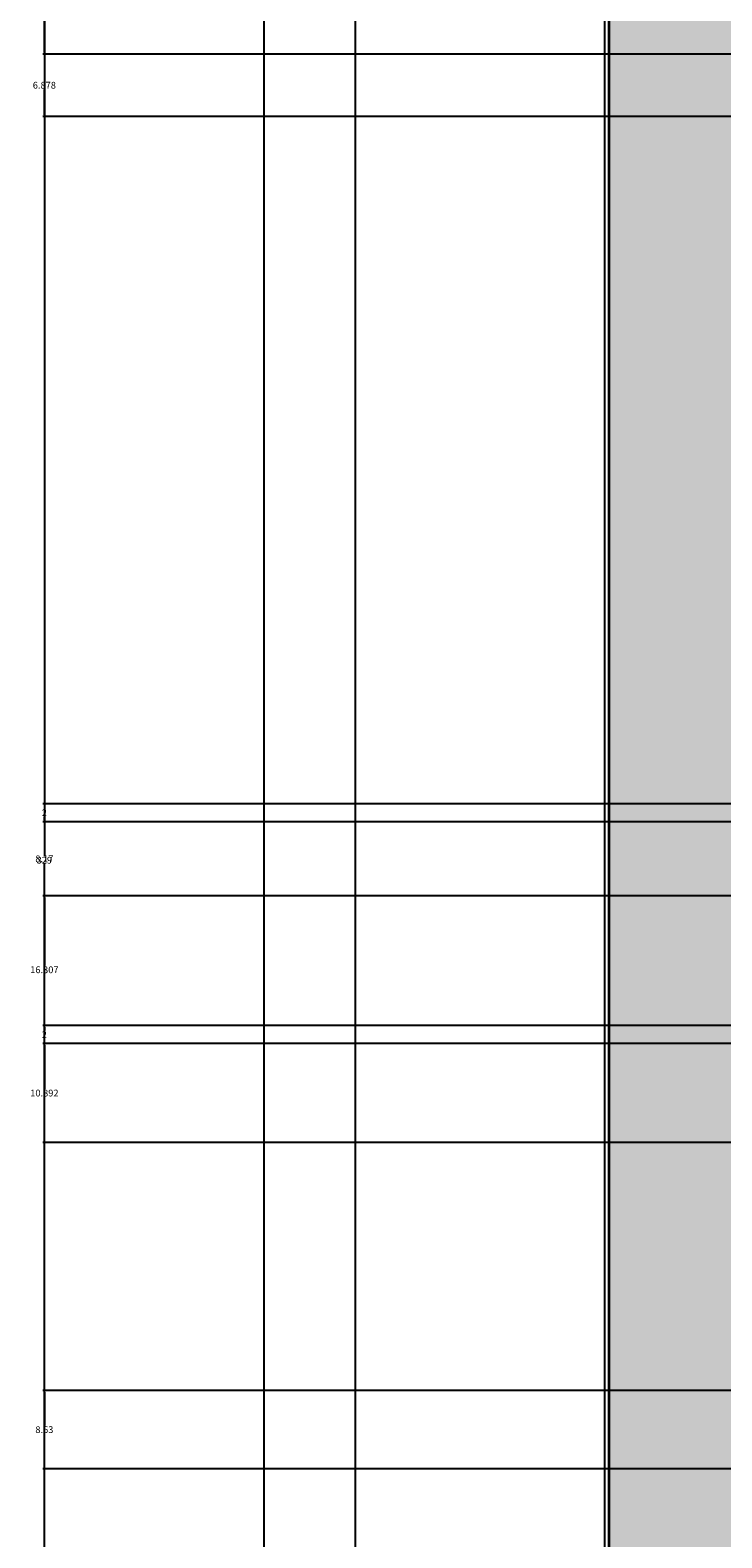
# Model space of a CAD drawing. Units: inches. Extents: x 62 to 566, y 66 to 528.
# Tile 5 of 20: x 62 to 138, y 264 to 430. Entities that reach past the tile are written whole.
import ezdxf

# ---------------------------------------------------------------- set-up
doc = ezdxf.new("R2010")
doc.units = ezdxf.units.IN
doc.header["$MEASUREMENT"] = 0
for name, color, linetype, lineweight in [('A-ANNO-DIMS', 2, 'Continuous', 18), ('A-ELEV', 7, 'Continuous', 35), ('A-WALL-PATT', 8, 'Continuous', 13)]:
    doc.layers.add(name, color=color, linetype=linetype, lineweight=lineweight)
doc.styles.get("Standard").update_dxf_attribs({"font": 'arial.ttf'})
doc.dimstyles.get("Standard").update_dxf_attribs({"dimtxt": 0.75, "dimasz": 0.18, "dimexe": 0.18, "dimexo": 0.0625, "dimgap": 0.09, "dimtad": 0, "dimtih": 1, "dimtoh": 1, "dimdec": 4, "dimzin": 0, "dimdsep": 46, "dimlunit": 4, "dimtxsty": 'Standard', "dimcen": 0.09, "dimadec": 0, "dimazin": 0, "dimtfac": 1, "dimtdec": 4, "dimtofl": 0, "dimtmove": 0, "dimatfit": 3, "dimfxl": 1, "dimtolj": 1, "dimtzin": 0, "dimarcsym": 0})

# ---------------------------------------------------------------- blocks, each defined once
blk = doc.blocks.new('*D8')
at = {"layer": 'A-ANNO-DIMS', "color": 0, "lineweight": -2, "transparency": 16777216}
for p, q in [((284.2, 271.35), (284.2, 65.94)), ((125.94, 126.31), (125.94, 65.94)), ((126.12, 66.12), (203.46, 66.12)), ((284.02, 66.12), (206.68, 66.12))]:
    blk.add_line(p, q, dxfattribs=at)
at = {"layer": 'A-ANNO-DIMS', "color": 0, "transparency": 16777216}
for points in [[(126.12, 66.15), (126.12, 66.09), (125.94, 66.12)], [(284.02, 66.15), (284.02, 66.09), (284.2, 66.12)]]:
    blk.add_solid(points, dxfattribs=at)
at = {"layer": 'Defpoints', "color": 0, "transparency": 16777216}
for p in [(284.2, 271.41), (125.94, 126.37), (284.2, 66.12)]:
    blk.add_point(p, dxfattribs=at)
at = {"layer": 'A-ANNO-DIMS', "color": 0, "transparency": 16777216, "insert": (205.07, 66.12), "char_height": 0.75, "attachment_point": 5}
blk.add_mtext('\\A1;158.26', dxfattribs=at)
blk = doc.blocks.new('*D14')
at = {"layer": 'A-ANNO-DIMS', "color": 0, "lineweight": -2, "transparency": 16777216}
for p, q in [((87.9, 174.13), (87.9, 527.47)), ((88.08, 527.29), (91.61, 527.29)), ((97.79, 527.29), (94.25, 527.29)), ((97.97, 174.13), (97.97, 527.47))]:
    blk.add_line(p, q, dxfattribs=at)
at = {"layer": 'A-ANNO-DIMS', "color": 0, "transparency": 16777216}
for points in [[(88.08, 527.32), (88.08, 527.26), (87.9, 527.29)], [(97.79, 527.32), (97.79, 527.26), (97.97, 527.29)]]:
    blk.add_solid(points, dxfattribs=at)
at = {"layer": 'Defpoints', "color": 0, "transparency": 16777216}
for p in [(97.97, 527.29), (87.9, 174.07), (97.97, 174.07)]:
    blk.add_point(p, dxfattribs=at)
at = {"layer": 'A-ANNO-DIMS', "color": 0, "transparency": 16777216, "insert": (92.93, 527.29), "char_height": 0.75, "attachment_point": 5}
blk.add_mtext('\\A1;10.07', dxfattribs=at)
blk = doc.blocks.new('*D15')
at = {"layer": 'A-ANNO-DIMS', "color": 0, "lineweight": -2, "transparency": 16777216}
for p, q in [((97.97, 174.13), (97.97, 527.47)), ((98.15, 527.29), (110.64, 527.29)), ((125.28, 527.29), (112.79, 527.29)), ((125.46, 174.13), (125.46, 527.47))]:
    blk.add_line(p, q, dxfattribs=at)
at = {"layer": 'A-ANNO-DIMS', "color": 0, "transparency": 16777216}
for points in [[(98.15, 527.32), (98.15, 527.26), (97.97, 527.29)], [(125.28, 527.32), (125.28, 527.26), (125.46, 527.29)]]:
    blk.add_solid(points, dxfattribs=at)
at = {"layer": 'Defpoints', "color": 0, "transparency": 16777216}
for p in [(125.46, 527.29), (97.97, 174.07), (125.46, 174.07)]:
    blk.add_point(p, dxfattribs=at)
at = {"layer": 'A-ANNO-DIMS', "color": 0, "transparency": 16777216, "insert": (111.72, 527.29), "char_height": 0.75, "attachment_point": 5}
blk.add_mtext('\\A1;27.5', dxfattribs=at)
blk = doc.blocks.new('*D18')
at = {"layer": 'A-ANNO-DIMS', "color": 0, "lineweight": -2, "transparency": 16777216}
for p, q in [((120.34, 503.04), (63.47, 503.04)), ((63.65, 502.86), (63.65, 339.03)), ((63.65, 174.25), (63.65, 338.08)), ((87.83, 174.07), (63.47, 174.07))]:
    blk.add_line(p, q, dxfattribs=at)
at = {"layer": 'A-ANNO-DIMS', "color": 0, "transparency": 16777216}
for points in [[(63.62, 502.86), (63.68, 502.86), (63.65, 503.04)], [(63.62, 174.25), (63.68, 174.25), (63.65, 174.07)]]:
    blk.add_solid(points, dxfattribs=at)
at = {"layer": 'Defpoints', "color": 0, "transparency": 16777216}
for p in [(63.65, 503.04), (120.41, 503.04), (87.9, 174.07)]:
    blk.add_point(p, dxfattribs=at)
at = {"layer": 'A-ANNO-DIMS', "color": 0, "transparency": 16777216, "insert": (63.65, 338.55), "char_height": 0.75, "attachment_point": 5}
blk.add_mtext('\\A1;329', dxfattribs=at)
blk = doc.blocks.new('*D35')
at = {"layer": 'A-ANNO-DIMS', "color": 0, "lineweight": -2, "transparency": 16777216}
for p, q in [((125.94, 461.98), (125.94, 65.94)), ((142.39, 445.04), (142.39, 65.94)), ((126.12, 66.12), (132.55, 66.12)), ((142.21, 66.12), (135.77, 66.12))]:
    blk.add_line(p, q, dxfattribs=at)
at = {"layer": 'A-ANNO-DIMS', "color": 0, "transparency": 16777216}
for points in [[(126.12, 66.15), (126.12, 66.09), (125.94, 66.12)], [(142.21, 66.15), (142.21, 66.09), (142.39, 66.12)]]:
    blk.add_solid(points, dxfattribs=at)
at = {"layer": 'Defpoints', "color": 0, "transparency": 16777216}
for p in [(125.94, 462.04), (142.39, 445.11), (142.39, 66.12)]:
    blk.add_point(p, dxfattribs=at)
at = {"layer": 'A-ANNO-DIMS', "color": 0, "transparency": 16777216, "insert": (134.16, 66.12), "char_height": 0.75, "attachment_point": 5}
blk.add_mtext('\\A1;16.443', dxfattribs=at)
blk = doc.blocks.new('*D44')
at = {"layer": 'A-ANNO-DIMS', "color": 0, "lineweight": -2, "transparency": 16777216}
for p, q in [((163.59, 427.48), (63.47, 427.48)), ((63.65, 427.3), (63.65, 424.51)), ((63.65, 420.78), (63.65, 423.56)), ((168.98, 420.6), (63.47, 420.6))]:
    blk.add_line(p, q, dxfattribs=at)
at = {"layer": 'A-ANNO-DIMS', "color": 0, "transparency": 16777216}
for points in [[(63.62, 427.3), (63.68, 427.3), (63.65, 427.48)], [(63.62, 420.78), (63.68, 420.78), (63.65, 420.6)]]:
    blk.add_solid(points, dxfattribs=at)
at = {"layer": 'Defpoints', "color": 0, "transparency": 16777216}
for p in [(63.65, 427.48), (163.65, 427.48), (169.04, 420.6)]:
    blk.add_point(p, dxfattribs=at)
at = {"layer": 'A-ANNO-DIMS', "color": 0, "transparency": 16777216, "insert": (63.65, 424.04), "char_height": 0.75, "attachment_point": 5}
blk.add_mtext('\\A1;6.878', dxfattribs=at)
blk = doc.blocks.new('*D45')
at = {"layer": 'A-ANNO-DIMS', "color": 0, "lineweight": -2, "transparency": 16777216}
for p, q in [((142.32, 445.11), (63.47, 445.11)), ((63.65, 444.93), (63.65, 436.76)), ((63.65, 427.66), (63.65, 435.82)), ((163.59, 427.48), (63.47, 427.48))]:
    blk.add_line(p, q, dxfattribs=at)
at = {"layer": 'A-ANNO-DIMS', "color": 0, "transparency": 16777216}
for points in [[(63.62, 444.93), (63.68, 444.93), (63.65, 445.11)], [(63.62, 427.66), (63.68, 427.66), (63.65, 427.48)]]:
    blk.add_solid(points, dxfattribs=at)
at = {"layer": 'Defpoints', "color": 0, "transparency": 16777216}
for p in [(63.65, 445.11), (142.39, 445.11), (163.65, 427.48)]:
    blk.add_point(p, dxfattribs=at)
at = {"layer": 'A-ANNO-DIMS', "color": 0, "transparency": 16777216, "insert": (63.65, 436.29), "char_height": 0.75, "attachment_point": 5}
blk.add_mtext('\\A1;17.63', dxfattribs=at)
blk = doc.blocks.new('*D98')
at = {"layer": 'A-ANNO-DIMS', "color": 0, "lineweight": -2, "transparency": 16777216}
for p, q in [((296.31, 280.04), (63.47, 280.04)), ((63.65, 279.86), (63.65, 276.2)), ((63.65, 271.59), (63.65, 275.25)), ((284.14, 271.41), (63.47, 271.41))]:
    blk.add_line(p, q, dxfattribs=at)
at = {"layer": 'A-ANNO-DIMS', "color": 0, "transparency": 16777216}
for points in [[(63.62, 279.86), (63.68, 279.86), (63.65, 280.04)], [(63.62, 271.59), (63.68, 271.59), (63.65, 271.41)]]:
    blk.add_solid(points, dxfattribs=at)
at = {"layer": 'Defpoints', "color": 0, "transparency": 16777216}
for p in [(63.65, 280.04), (296.38, 280.04), (284.2, 271.41)]:
    blk.add_point(p, dxfattribs=at)
at = {"layer": 'A-ANNO-DIMS', "color": 0, "transparency": 16777216, "insert": (63.65, 275.73), "char_height": 0.75, "attachment_point": 5}
blk.add_mtext('\\A1;8.63', dxfattribs=at)
blk = doc.blocks.new('*D99')
at = {"layer": 'A-ANNO-DIMS', "color": 0, "lineweight": -2, "transparency": 16777216}
for p, q in [((284.14, 318.31), (63.47, 318.31)), ((63.65, 318.13), (63.65, 313.33)), ((63.65, 307.59), (63.65, 312.39)), ((284.14, 307.41), (63.47, 307.41))]:
    blk.add_line(p, q, dxfattribs=at)
at = {"layer": 'A-ANNO-DIMS', "color": 0, "transparency": 16777216}
for points in [[(63.62, 318.13), (63.68, 318.13), (63.65, 318.31)], [(63.62, 307.59), (63.68, 307.59), (63.65, 307.41)]]:
    blk.add_solid(points, dxfattribs=at)
at = {"layer": 'Defpoints', "color": 0, "transparency": 16777216}
for p in [(63.65, 318.31), (284.2, 318.31), (284.2, 307.41)]:
    blk.add_point(p, dxfattribs=at)
at = {"layer": 'A-ANNO-DIMS', "color": 0, "transparency": 16777216, "insert": (63.65, 312.86), "char_height": 0.75, "attachment_point": 5}
blk.add_mtext('\\A1;10.892', dxfattribs=at)
blk = doc.blocks.new('*D100')
at = {"layer": 'A-ANNO-DIMS', "color": 0, "lineweight": -2, "transparency": 16777216}
for p, q in [((284.14, 334.61), (63.47, 334.61)), ((63.65, 334.43), (63.65, 326.93)), ((63.65, 318.49), (63.65, 325.99)), ((284.14, 318.31), (63.47, 318.31))]:
    blk.add_line(p, q, dxfattribs=at)
at = {"layer": 'A-ANNO-DIMS', "color": 0, "transparency": 16777216}
for points in [[(63.62, 334.43), (63.68, 334.43), (63.65, 334.61)], [(63.62, 318.49), (63.68, 318.49), (63.65, 318.31)]]:
    blk.add_solid(points, dxfattribs=at)
at = {"layer": 'Defpoints', "color": 0, "transparency": 16777216}
for p in [(63.65, 334.61), (284.2, 334.61), (284.2, 318.31)]:
    blk.add_point(p, dxfattribs=at)
at = {"layer": 'A-ANNO-DIMS', "color": 0, "transparency": 16777216, "insert": (63.65, 326.46), "char_height": 0.75, "attachment_point": 5}
blk.add_mtext('\\A1;16.307', dxfattribs=at)
blk = doc.blocks.new('*D101')
at = {"layer": 'A-ANNO-DIMS', "color": 0, "lineweight": -2, "transparency": 16777216}
for p, q in [((284.14, 342.78), (63.47, 342.78)), ((63.65, 342.6), (63.65, 339.17)), ((63.65, 334.79), (63.65, 338.22)), ((284.14, 334.61), (63.47, 334.61))]:
    blk.add_line(p, q, dxfattribs=at)
at = {"layer": 'A-ANNO-DIMS', "color": 0, "transparency": 16777216}
for points in [[(63.62, 342.6), (63.68, 342.6), (63.65, 342.78)], [(63.62, 334.79), (63.68, 334.79), (63.65, 334.61)]]:
    blk.add_solid(points, dxfattribs=at)
at = {"layer": 'Defpoints', "color": 0, "transparency": 16777216}
for p in [(63.65, 342.78), (284.2, 342.78), (284.2, 334.61)]:
    blk.add_point(p, dxfattribs=at)
at = {"layer": 'A-ANNO-DIMS', "color": 0, "transparency": 16777216, "insert": (63.65, 338.7), "char_height": 0.75, "attachment_point": 5}
blk.add_mtext('\\A1;8.17', dxfattribs=at)
blk = doc.blocks.new('*D102')
at = {"layer": 'A-ANNO-DIMS', "color": 0, "lineweight": -2, "transparency": 16777216}
for p, q in [((284.14, 344.78), (63.47, 344.78)), ((63.65, 344.6), (63.65, 344.25)), ((284.14, 342.78), (63.47, 342.78)), ((63.65, 342.96), (63.65, 343.32))]:
    blk.add_line(p, q, dxfattribs=at)
at = {"layer": 'A-ANNO-DIMS', "color": 0, "transparency": 16777216}
for points in [[(63.62, 344.6), (63.68, 344.6), (63.65, 344.78)], [(63.62, 342.96), (63.68, 342.96), (63.65, 342.78)]]:
    blk.add_solid(points, dxfattribs=at)
at = {"layer": 'Defpoints', "color": 0, "transparency": 16777216}
for p in [(63.65, 344.78), (284.2, 344.78), (284.2, 342.78)]:
    blk.add_point(p, dxfattribs=at)
at = {"layer": 'A-ANNO-DIMS', "color": 0, "transparency": 16777216, "insert": (63.65, 343.78), "char_height": 0.75, "attachment_point": 5}
blk.add_mtext('\\A1;2', dxfattribs=at)
blk = doc.blocks.new('*D103')
at = {"layer": 'A-ANNO-DIMS', "color": 0, "lineweight": -2, "transparency": 16777216}
for p, q in [((284.14, 320.31), (63.47, 320.31)), ((63.65, 320.13), (63.65, 319.77)), ((284.14, 318.31), (63.47, 318.31)), ((63.65, 318.49), (63.65, 318.84))]:
    blk.add_line(p, q, dxfattribs=at)
at = {"layer": 'A-ANNO-DIMS', "color": 0, "transparency": 16777216}
for points in [[(63.62, 320.13), (63.68, 320.13), (63.65, 320.31)], [(63.62, 318.49), (63.68, 318.49), (63.65, 318.31)]]:
    blk.add_solid(points, dxfattribs=at)
at = {"layer": 'Defpoints', "color": 0, "transparency": 16777216}
for p in [(63.65, 320.31), (284.2, 320.31), (284.2, 318.31)]:
    blk.add_point(p, dxfattribs=at)
at = {"layer": 'A-ANNO-DIMS', "color": 0, "transparency": 16777216, "insert": (63.65, 319.31), "char_height": 0.75, "attachment_point": 5}
blk.add_mtext('\\A1;2', dxfattribs=at)
blk = doc.blocks.new('*D130')
at = {"layer": 'A-ANNO-DIMS', "color": 0, "lineweight": -2, "transparency": 16777216}
for p, q in [((227.74, 280.04), (63.47, 280.04)), ((63.65, 279.86), (63.65, 276.2)), ((63.65, 271.59), (63.65, 275.25)), ((217.21, 271.41), (63.47, 271.41))]:
    blk.add_line(p, q, dxfattribs=at)
at = {"layer": 'A-ANNO-DIMS', "color": 0, "transparency": 16777216}
for points in [[(63.62, 279.86), (63.68, 279.86), (63.65, 280.04)], [(63.62, 271.59), (63.68, 271.59), (63.65, 271.41)]]:
    blk.add_solid(points, dxfattribs=at)
at = {"layer": 'Defpoints', "color": 0, "transparency": 16777216}
for p in [(63.65, 280.04), (227.8, 280.04), (217.28, 271.41)]:
    blk.add_point(p, dxfattribs=at)
at = {"layer": 'A-ANNO-DIMS', "color": 0, "transparency": 16777216, "insert": (63.65, 275.73), "char_height": 0.75, "attachment_point": 5}
blk.add_mtext('\\A1;8.63', dxfattribs=at)

msp = doc.modelspace()

# ---------------------------------------------------------------- hatches: boundary and pattern name
at = {"layer": 'A-WALL-PATT'}
h = msp.add_hatch(color=256, dxfattribs=at)
h.dxf.hatch_style = 1
h.paths.add_polyline_path([(416.0836, 462.0423), (125.9418, 462.0423), (125.9418, 414.3686), (125.9418, 270.3686), (125.9418, 126.3686), (142.3851, 126.3686), (142.3851, 270.3686), (142.3851, 414.3686), (142.3851, 445.1064), (284.2021, 445.1064), (416.0836, 445.1064)])
h.paths.add_polyline_path([(435.3945, 503.0423), (426.3652, 503.0423), (120.4058, 503.0423), (120.4058, 501.0423), (125.9418, 501.0423), (416.0836, 501.0423), (426.3652, 501.0423), (430.6938, 501.0423), (435.3945, 501.0423)])
h.paths.add_polyline_path([(439.6878, 352.4848), (392.4793, 352.4848), (392.4793, 307.4128), (217.2752, 307.4128), (217.2752, 295.4098), (217.2752, 271.4128), (272.0586, 271.4128), (439.6878, 271.4128)])
h.paths.add_polyline_path([(248.0143, 297.1682), (255.6783, 297.1682), (255.6783, 280.0423), (248.0143, 280.0423)], flags=16)
h.paths.add_polyline_path([(235.4641, 280.0423), (227.8001, 280.0423), (227.8001, 297.1682), (235.4641, 297.1682)], flags=16)
h.paths.add_polyline_path([(270.4427, 297.1682), (278.1067, 297.1682), (278.1067, 280.0423), (270.4427, 280.0423)], flags=16)
h.paths.add_polyline_path([(296.3755, 297.1682), (304.0395, 297.1682), (304.0395, 280.0423), (296.3755, 280.0423)], flags=16)
h.paths.add_polyline_path([(319.2543, 297.1682), (326.9183, 297.1682), (326.9183, 280.0423), (319.2543, 280.0423)], flags=16)
h.paths.add_polyline_path([(341.2622, 297.1682), (348.9262, 297.1682), (348.9262, 280.0423), (341.2622, 280.0423)], flags=16)
h.paths.add_polyline_path([(389.2857, 298.3985), (433.8102, 298.3985), (433.8102, 294.9497), (389.2857, 294.9497)], flags=16)
h.paths.add_polyline_path([(389.2857, 291.6038), (433.8102, 291.6038), (433.8102, 288.155), (389.2857, 288.155)], flags=16)
h.paths.add_polyline_path([(389.2857, 284.9607), (433.8102, 284.9607), (433.8102, 281.5119), (389.2857, 281.5119)], flags=16)
h.paths.add_polyline_path([(403.5849, 311.4736), (403.5849, 317.4388), (433.1636, 317.4388), (433.1636, 311.4736)], flags=16)
h.paths.add_polyline_path([(403.5849, 323.1329), (403.5849, 329.0982), (433.1636, 329.0982), (433.1636, 323.1329)], flags=16)
h.paths.add_polyline_path([(403.5849, 334.5211), (403.5849, 340.4863), (433.1636, 340.4863), (433.1636, 334.5211)], flags=16)
h.paths.add_polyline_path([(272.0586, 160.3545), (217.2752, 160.3545), (217.2752, 129.0504), (217.2752, 126.3686), (272.0586, 126.3686)], flags=17)
h.paths.add_polyline_path([(220.5897, 149.5749), (220.5897, 152.296), (267.7931, 152.296), (267.7931, 149.5749)], flags=16)
h.paths.add_polyline_path([(267.7931, 146.6724), (267.7931, 143.9513), (220.5897, 143.9513), (220.5897, 146.6724)], flags=16)
h.paths.add_polyline_path([(220.5897, 155.3799), (220.5897, 158.101), (267.7931, 158.101), (267.7931, 155.3799)], flags=16)
h.paths.add_polyline_path([(267.7931, 140.686), (267.7931, 137.9649), (220.5897, 137.9649), (220.5897, 140.686)], flags=16)
h.paths.add_polyline_path([(267.7931, 135.516), (267.7931, 132.7949), (220.5897, 132.7949), (220.5897, 135.516)], flags=16)

# ---------------------------------------------------------------- linework, layer by layer
at = {"layer": 'A-ELEV'}
for p, q in [((125.9418, 414.3686), (125.9418, 462.0423)), ((125.9418, 270.3686), (125.9418, 414.3686)), ((125.9418, 126.3686), (125.9418, 270.3686))]:
    msp.add_line(p, q, dxfattribs=at)

# ---------------------------------------------------------------- dimensions: what is measured, and where the dimension line sits
at = {"layer": 'A-ANNO-DIMS'}
for base, p1, p2, override, picture, middle in [((97.967, 527.2923), (87.8962, 174.0659), (97.967, 174.0659), {"dimdec": 2, "dimlfac": 1, "dimrnd": 0, "dimzin": 0, "dimdsep": 46, "dimlunit": 2}, '*D14', (92.9316, 527.2923)), ((125.4645, 527.2923), (97.967, 174.0659), (125.4645, 174.0659), {"dimdec": 1, "dimlfac": 1, "dimrnd": 0, "dimzin": 0, "dimdsep": 46, "dimlunit": 2}, '*D15', (111.7157, 527.2923)), ((142.3851, 66.1186), (125.9418, 462.0423), (142.3851, 445.1064), {"dimdec": 3, "dimlfac": 1, "dimrnd": 0, "dimzin": 0, "dimdsep": 46, "dimlunit": 2}, '*D35', (134.1634, 66.1186)), ((284.2021, 66.1186), (125.9418, 126.3686), (284.2021, 271.4128), {"dimdec": 2, "dimlfac": 1, "dimrnd": 0, "dimzin": 0, "dimdsep": 46, "dimlunit": 2}, '*D8', (205.0719, 66.1186))]:
    dim = msp.add_linear_dim(base=base, p1=p1, p2=p2, dimstyle='Standard', override=override, dxfattribs=at)
    dim.commit()
    dim.dimension.update_dxf_attribs({"geometry": picture, "text_midpoint": middle})
for base, p1, p2, override, picture, middle in [((63.6462, 503.0423), (87.8962, 174.0659), (120.4058, 503.0423), {"dimdec": 0, "dimlfac": 1, "dimrnd": 0, "dimzin": 0, "dimdsep": 46, "dimlunit": 2}, '*D18', (63.6462, 338.5541)), ((63.6462, 445.1064), (163.6548, 427.4752), (142.3851, 445.1064), {"dimdec": 2, "dimlfac": 1, "dimrnd": 0, "dimzin": 0, "dimdsep": 46, "dimlunit": 2}, '*D45', (63.6462, 436.2908)), ((63.6462, 427.4752), (169.0431, 420.597), (163.6548, 427.4752), {"dimdec": 3, "dimlfac": 1, "dimrnd": 0, "dimzin": 0, "dimdsep": 46, "dimlunit": 2}, '*D44', (63.6462, 424.0361)), ((63.6462, 344.7821), (284.2021, 342.7821), (284.2021, 344.7821), {"dimdec": 0, "dimlfac": 1, "dimrnd": 0, "dimzin": 0, "dimdsep": 46, "dimlunit": 2}, '*D102', (63.6462, 343.7821)), ((63.6462, 342.7821), (284.2021, 334.6119), (284.2021, 342.7821), {"dimdec": 2, "dimlfac": 1, "dimrnd": 0, "dimzin": 0, "dimdsep": 46, "dimlunit": 2}, '*D101', (63.6462, 338.697)), ((63.6462, 334.6119), (284.2021, 318.3051), (284.2021, 334.6119), {"dimdec": 3, "dimlfac": 1, "dimrnd": 0, "dimzin": 0, "dimdsep": 46, "dimlunit": 2}, '*D100', (63.6462, 326.4585)), ((63.6462, 320.3051), (284.2021, 318.3051), (284.2021, 320.3051), {"dimdec": 0, "dimlfac": 1, "dimrnd": 0, "dimzin": 0, "dimdsep": 46, "dimlunit": 2}, '*D103', (63.6462, 319.3051)), ((63.6462, 318.3051), (284.2021, 307.4128), (284.2021, 318.3051), {"dimdec": 3, "dimlfac": 1, "dimrnd": 0, "dimzin": 0, "dimdsep": 46, "dimlunit": 2}, '*D99', (63.6462, 312.8589)), ((63.6462, 280.0423), (284.2021, 271.4128), (296.3755, 280.0423), {"dimdec": 2, "dimlfac": 1, "dimrnd": 0, "dimzin": 0, "dimdsep": 46, "dimlunit": 2}, '*D98', (63.6462, 275.7276)), ((63.6462, 280.0423), (217.2752, 271.4128), (227.8001, 280.0423), {"dimdec": 2, "dimlfac": 1, "dimrnd": 0, "dimzin": 0, "dimdsep": 46, "dimlunit": 2}, '*D130', (63.6462, 275.7276))]:
    dim = msp.add_linear_dim(base=base, p1=p1, p2=p2, angle=90, dimstyle='Standard', override=override, dxfattribs=at)
    dim.commit()
    dim.dimension.update_dxf_attribs({"geometry": picture, "text_midpoint": middle})

doc.saveas('drawing.dxf')
